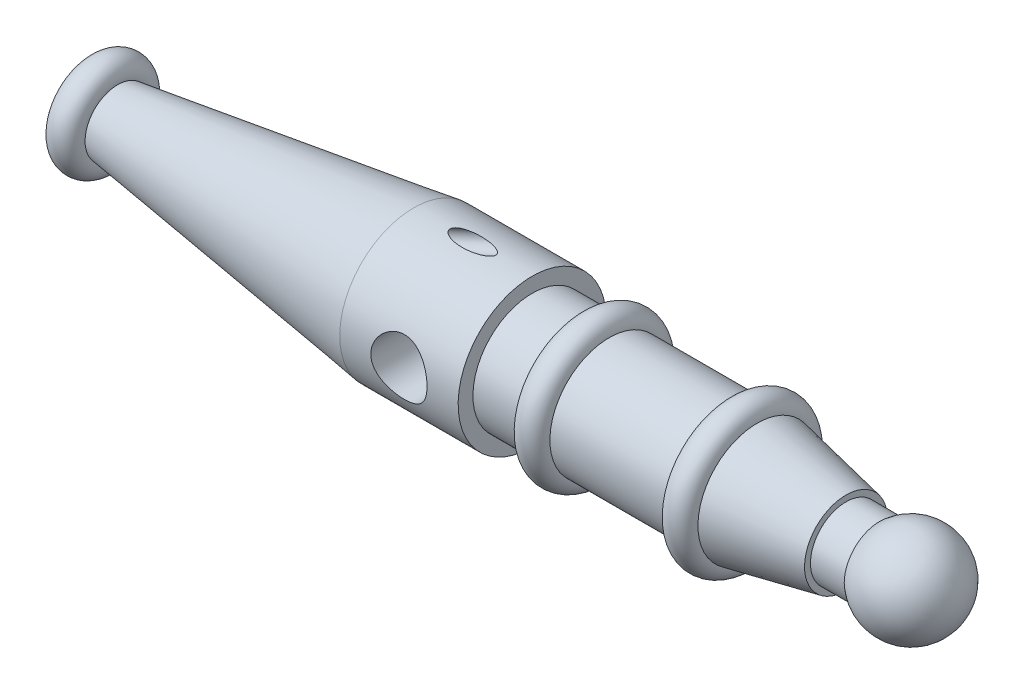
SolidWorks part; units mm, degrees
material "Plain Carbon Steel"
ref_plane "Front Plane" through (0, 0, 0) normal (0, 0, 1) x (1, 0, 0)
ref_plane "Top Plane" through (0, 0, 0) normal (0, 1, 0) x (1, 0, 0)
ref_plane "Right Plane" through (0, 0, 0) normal (1, 0, 0) x (0, 0, -1)
sketch "Body Profile Sketch" plane through (0, 0, 0) normal (0, 0, 1) x (1, 0, 0)
  line L0 (-676.8322, 0) -> (793.0828, 0) construction
  line L1 (-676.8322, 55) -> (-676.8322, 0)
  line L2 (73.1678, 125) -> (73.1678, 100)
  line L3 (-126.8322, 125) -> (73.1678, 125)
  line L4 (-626.8322, 55) -> (-126.8322, 125)
  line L5 (73.1678, 100) -> (153.1678, 100)
  line L6 (203.1678, 100) -> (403.1678, 100)
  line L7 (453.1678, 100) -> (603.1678, 70)
  line L8 (603.1678, 70) -> (603.1678, 60)
  line L9 (603.1678, 60) -> (660.1678, 60)
  line L10 (-676.8322, 0) -> (793.0828, 0)
  arc A0 (-676.8322, 55) -> (-626.8322, 55) centre (-651.8322, 60) cw
  arc A1 (153.1678, 100) -> (203.1678, 100) centre (178.1678, 100) cw
  arc A2 (403.1678, 100) -> (453.1678, 100) centre (428.1678, 100) cw
  arc A4 (793.0828, 0) -> (660.1678, 60) centre (713.0828, 0) ccw
  dimension "D4" = 25
  dimension "D8" = 25
  dimension "D13" = 676.8322
  dimension "120" = 160
  dimension "D1" = 100
  dimension "D2" = 55
  dimension "D3" = 830
  dimension "47.5" = 55
  dimension "750" = 750
  dimension "D5" = 50
  dimension "D6" = 1080
  dimension "D7" = 50
  dimension "D9" = 70
  dimension "D10" = 1280
  dimension "D11" = 60
  dimension "D12" = 57
  dimension "D14" = 50
  dimension "D15" = 125
  dimension "D16" = 200
revolve "Revolved Body" add sketch "Body Profile Sketch" angle 360 about L0
sketch "Bore Sketch Ø64" plane through (-676.8322, 0, 0) normal (-1, 0, 0) x (0, 0, 1)
  circle A0 centre (0, 0) radius 32
  dimension "D1" = 64
extrude "Bore Ø64 x375" cut sketch "Bore Sketch Ø64" against normal blind 375
chamfer "Bore Mouth Chamfer 16x45" distance 16 angle 45 1 edges at (-676.8322, -32, 0)
sketch "Cross Hole Sketch" plane through (0, 0, 0) normal (0, 0, 1) x (1, 0, 0)
  line L0 (-26.8322, 125) -> (-26.8322, -125) construction
  line L1 (73.1678, 125) -> (-126.8322, 125) construction
  line L2 (-126.8322, -125) -> (73.1678, -125) construction
  circle A0 centre (-26.8322, 0) radius 47.5
  point P8 (-26.8322, 0)
  dimension "D1" = 95
extrude "Cross Hole Cut" cut sketch "Cross Hole Sketch" against normal through all both and the other way through all
sketch "Groove Profile Sketch" plane through (0, 0, 0) normal (0, 0, 1) x (1, 0, 0)
  line L0 (-350.038, -5.0867) -> (-343.3886, -19.6395)
  line L2 (-343.3886, -19.6395) -> (28.843, 150.4389)
  line L3 (-343.3886, -19.6395) -> (28.843, 150.4389) construction
  line L4 (22.1936, 164.9917) -> (-350.038, -5.0867)
  line L6 (22.1936, 164.9917) -> (28.843, 150.4389)
  dimension "D1" = 409.2469
  dimension "D2" = 16
  dimension "D3" = 170.0784
  dimension "D4" = 343.3886
  dimension "D5" = 19.6395
revolve "Revolved Groove Cut" cut sketch "Groove Profile Sketch" angle 360 about L3
sketch "Deep Bore Sketch" plane through (-676.8322, 0, 0) normal (-1, 0, 0) x (0, 0, 1)
  circle A2 centre (0, 0) radius 32 construction
  circle A3 centre (0, 0) radius 32
extrude "Deep Bore Cut 555" cut sketch "Deep Bore Sketch" against normal blind 555
